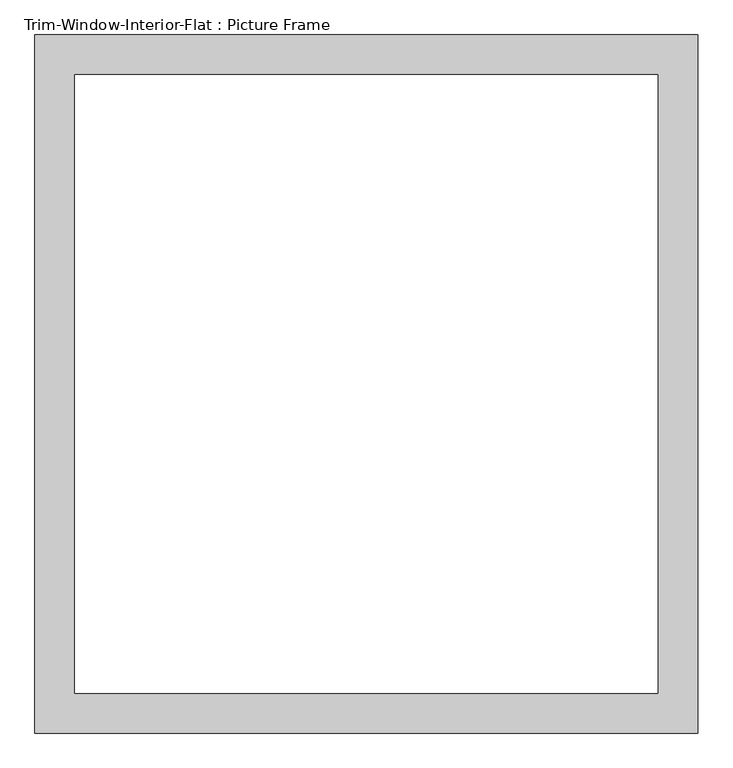
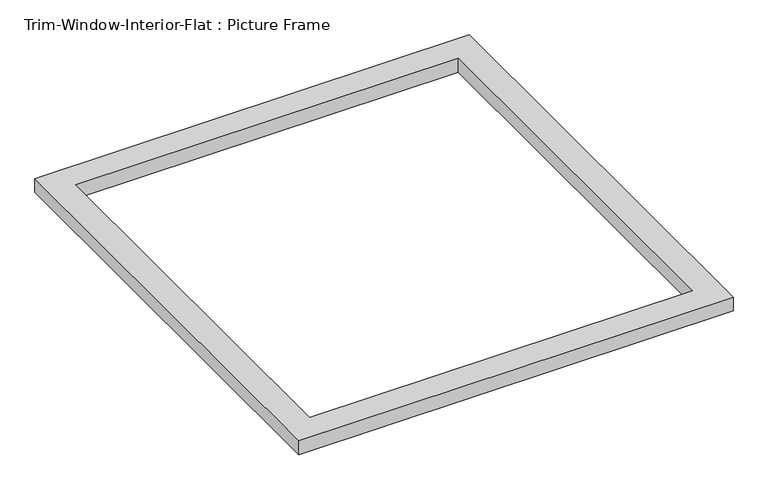
"""IFC4 building model written with IfcOpenShell, lengths in millimetres: proxy geometry, Trim-Window-Interior-Flat : Picture Frame."""

from ifc_helpers import new_model, si_unit, origin, origin_with_axes, place, context, project, spatial, polyline, outline, extrude, source, transform, mapped, element, save


def trim_window_interior_flat_picture_frame_51c85655(model_context):
    return source(origin(), model_context, "Body", "SweptSolid", [
        extrude(outline(polyline([(476.25, 44.45), (476.25, -958.85), (-476.25, -958.85), (-476.25, 44.45), (476.25, 44.45)]), holes=[polyline([(419.1, -12.7), (-419.1, -12.7), (-419.1, -901.7), (419.1, -901.7), (419.1, -12.7)])]), origin_with_axes(), (0.0, 0.0, 1.0), 31.75),
    ])


if __name__ == "__main__":
    model = new_model("IFC4")
    model_context = context("Model", 3, world=origin())
    ifc_project = project(units=[si_unit("LENGTHUNIT", "METRE", prefix="MILLI")], contexts=[model_context])
    site = spatial("IfcSite", under=ifc_project)
    building = spatial("IfcBuilding", under=site)
    placement = place(None, origin())
    trim_window_interior_flat_picture_frame_shape = trim_window_interior_flat_picture_frame_51c85655(model_context)
    element("IfcBuildingElementProxy", 1, Name="Trim-Window-Interior-Flat : Picture Frame", ObjectType="Trim-Window-Interior-Flat : Picture Frame", at=placement, inside=building, context=model_context, shape_type="MappedRepresentation", body=[
        mapped(trim_window_interior_flat_picture_frame_shape, transform((0.0, 0.0, 0.0), x_axis=(1.0, 0.0, 0.0), y_axis=(0.0, 1.0, 0.0), z_axis=(0.0, 0.0, 1.0))),
    ])
    save(model, "model.ifc")

# Revit data of these elements
# Type "Trim-Window-Interior-Flat : Picture Frame"
#   Trim Thickness_Picture Frame = 0.104167 ft
#   Trim Width = 0.1875 ft
#   Trim Thickness_with Sill = 0.0625 ft
#   Sill Thickness = 0.104167 ft
#   Opening Width [instance default] = 2 ft
#   Opening Height [instance default] = 3 ft
#   Default Elevation = 4 ft
#   Sill = no
#   Picture Frame = yes
#   Trim Material [instance default] = none
# Element 1 (IfcBuildingElementProxy, "Trim-Window-Interior-Flat : Picture Frame")
#   Opening Width = 2.833333 ft
#   Trim Material = Wood - Stained
#   Materials on its faces: "Wood - Stained"
# Materials
#   "Wood - Stained": class "Wood", colour RGB 224 178 126, transparency 0, Cost = 0
